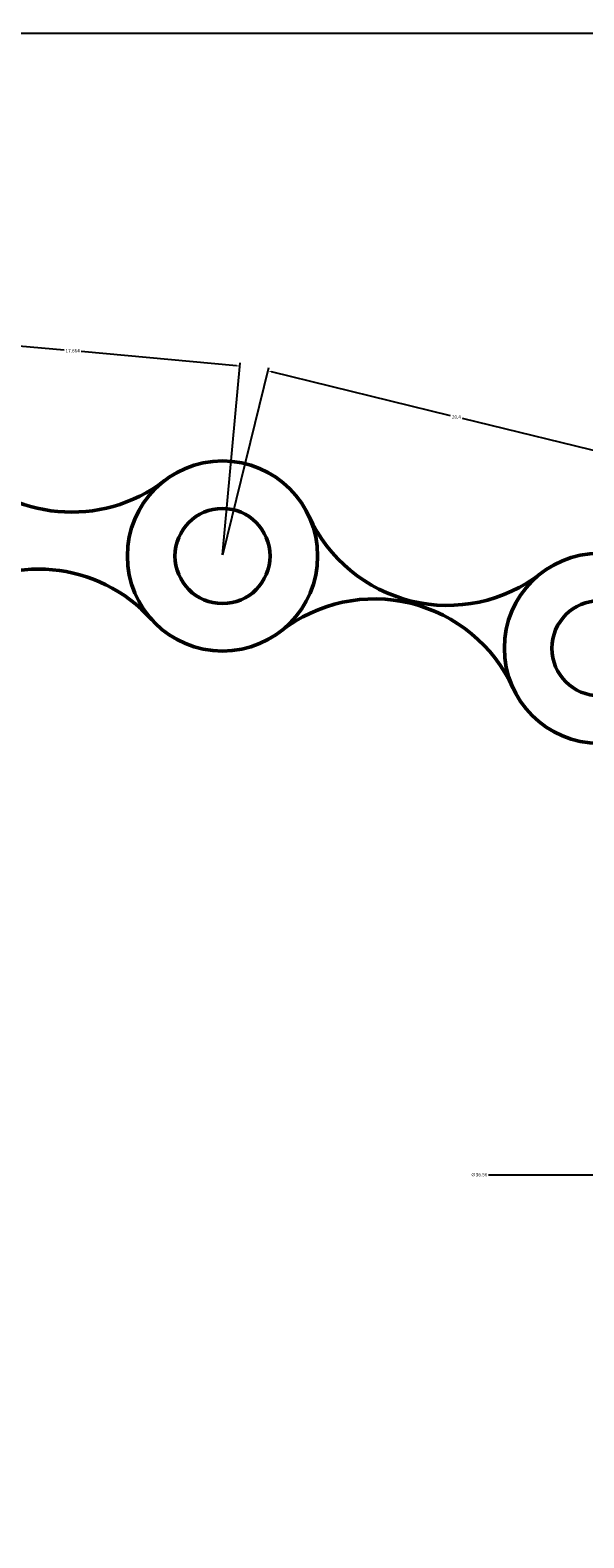
# Model space of a CAD drawing. Units: inches. Extents: x 413 to 622, y 326 to 447.
# Tile 11 of 15: x 539 to 568, y 367 to 447. Entities that reach past the tile are written whole.
import ezdxf

# ---------------------------------------------------------------- set-up
doc = ezdxf.new("R2010")
doc.units = ezdxf.units.IN
doc.header["$MEASUREMENT"] = 0
doc.layers.add('M-DIMS', color=2, linetype='Continuous', lineweight=18)
doc.layers.add('M-OUTL', color=7, linetype='Continuous', lineweight=50)
doc.styles.get("Standard").update_dxf_attribs({"font": 'arial.ttf'})
doc.dimstyles.get("Standard").update_dxf_attribs({"dimtxt": 0.18, "dimasz": 0.18, "dimexe": 0.18, "dimexo": 0.0625, "dimgap": 0.09, "dimtad": 0, "dimtih": 1, "dimtoh": 1, "dimdec": 4, "dimzin": 0, "dimdsep": 46, "dimtxsty": 'Standard', "dimcen": 0.09, "dimadec": 0, "dimazin": 0, "dimtfac": 1, "dimtdec": 4, "dimtofl": 0, "dimtmove": 0, "dimatfit": 3, "dimfxl": 1, "dimtolj": 1, "dimtzin": 0, "dimarcsym": 0})

# ---------------------------------------------------------------- blocks, each defined once
blk = doc.blocks.new('CHAIN-ROLLER-PIN')
for radius in [5, 2.5]:
    blk.add_circle((5, 5), radius)
blk = doc.blocks.new('CHAIN-LINK-WAIST-P17_664')
for centre, start, end in [((6.624, 13.651), 221.93853, 307.52912), ((4.873, -5.347), 41.93853, 127.52912)]:
    blk.add_arc(centre, 8, start, end)
blk = doc.blocks.new('CHAIN-LINK-WAIST-P20_400')
for centre, start, end in [((8.752, 12.333), 204.55472, 307.92191), ((4.917, -3.325), 24.55472, 127.92191)]:
    blk.add_arc(centre, 8, start, end)
blk = doc.blocks.new('*D11')
at = {"layer": 'Defpoints', "color": 0, "transparency": 16777216}
for p in [(621.66, 446.422), (621.66, 388.074), (423.314, 378.888)]:
    blk.add_point(p, dxfattribs=at)
at = {"layer": 'M-DIMS', "color": 0, "lineweight": -2, "transparency": 16777216}
for p, q in [((423.314, 378.95), (423.314, 446.602)), ((621.66, 388.137), (621.66, 446.602)), ((423.494, 446.422), (522.031, 446.422)), ((621.48, 446.422), (522.943, 446.422))]:
    blk.add_line(p, q, dxfattribs=at)
at = {"layer": 'M-DIMS', "color": 0, "transparency": 16777216}
for points in [[(423.494, 446.452), (423.494, 446.392), (423.314, 446.422)], [(621.48, 446.452), (621.48, 446.392), (621.66, 446.422)]]:
    blk.add_solid(points, dxfattribs=at)
at = {"layer": 'M-DIMS', "color": 0, "transparency": 16777216, "insert": (522.487, 446.422), "char_height": 0.18, "attachment_point": 5}
blk.add_mtext('\\A1;198.35', dxfattribs=at)
blk = doc.blocks.new('*D12')
at = {"layer": 'Defpoints', "color": 0, "transparency": 16777216}
for p in [(472.684, 386.392), (592.684, 386.392), (592.684, 326.361)]:
    blk.add_point(p, dxfattribs=at)
at = {"layer": 'M-DIMS', "color": 0, "lineweight": -2, "transparency": 16777216}
for p, q in [((472.684, 386.329), (472.684, 326.181)), ((592.684, 386.329), (592.684, 326.181)), ((472.864, 326.361), (532.404, 326.361)), ((592.504, 326.361), (532.964, 326.361))]:
    blk.add_line(p, q, dxfattribs=at)
at = {"layer": 'M-DIMS', "color": 0, "transparency": 16777216}
for points in [[(472.864, 326.391), (472.864, 326.331), (472.684, 326.361)], [(592.504, 326.391), (592.504, 326.331), (592.684, 326.361)]]:
    blk.add_solid(points, dxfattribs=at)
at = {"layer": 'M-DIMS', "color": 0, "transparency": 16777216, "insert": (532.684, 326.361), "char_height": 0.18, "attachment_point": 5}
blk.add_mtext('\\A1;120', dxfattribs=at)
blk = doc.blocks.new('*D20')
at = {"layer": 'Defpoints', "color": 0, "transparency": 16777216}
for p in [(550.373, 428.926), (531.863, 420.559), (549.452, 418.938)]:
    blk.add_point(p, dxfattribs=at)
at = {"layer": 'M-DIMS', "color": 0, "lineweight": -2, "transparency": 16777216}
for p, q in [((531.869, 420.621), (532.8, 430.726)), ((532.963, 430.53), (541.124, 429.778)), ((550.194, 428.942), (542.033, 429.694)), ((549.458, 419), (550.39, 429.105))]:
    blk.add_line(p, q, dxfattribs=at)
at = {"layer": 'M-DIMS', "color": 0, "transparency": 16777216}
for points in [[(532.966, 430.56), (532.96, 430.501), (532.784, 430.547)], [(550.197, 428.972), (550.191, 428.912), (550.373, 428.926)]]:
    blk.add_solid(points, dxfattribs=at)
at = {"layer": 'M-DIMS', "color": 0, "transparency": 16777216, "insert": (541.578, 429.736), "char_height": 0.18, "attachment_point": 5}
blk.add_mtext('\\A1;17.664', dxfattribs=at)
blk = doc.blocks.new('*D21')
at = {"layer": 'Defpoints', "color": 0, "transparency": 16777216}
for p in [(571.652, 423.827), (549.452, 418.938), (569.266, 414.085)]:
    blk.add_point(p, dxfattribs=at)
at = {"layer": 'M-DIMS', "color": 0, "lineweight": -2, "transparency": 16777216}
for p, q in [((549.467, 418.998), (551.881, 428.855)), ((552.013, 428.637), (561.421, 426.333)), ((571.478, 423.87), (562.07, 426.174)), ((569.281, 414.145), (571.695, 424.002))]:
    blk.add_line(p, q, dxfattribs=at)
at = {"layer": 'M-DIMS', "color": 0, "transparency": 16777216}
for points in [[(552.02, 428.666), (552.006, 428.608), (551.838, 428.68)], [(571.485, 423.899), (571.47, 423.841), (571.652, 423.827)]]:
    blk.add_solid(points, dxfattribs=at)
at = {"layer": 'M-DIMS', "color": 0, "transparency": 16777216, "insert": (561.745, 426.254), "char_height": 0.18, "attachment_point": 5}
blk.add_mtext('\\A1;20.4', dxfattribs=at)
blk = doc.blocks.new('*D25')
at = {"layer": 'Defpoints', "color": 0, "transparency": 16777216}
for p in [(574.404, 386.392), (610.964, 386.391)]:
    blk.add_point(p, dxfattribs=at)
at = {"layer": 'M-DIMS', "color": 0, "lineweight": -2, "transparency": 16777216}
for p, q in [((563.436, 386.392), (574.224, 386.392)), ((592.594, 386.392), (592.774, 386.392)), ((592.684, 386.302), (592.684, 386.482))]:
    blk.add_line(p, q, dxfattribs=at)
at = {"layer": 'M-DIMS', "color": 0, "transparency": 16777216}
blk.add_solid([(574.224, 386.422), (574.224, 386.362), (574.404, 386.392)], dxfattribs=at)
at = {"layer": 'M-DIMS', "color": 0, "transparency": 16777216, "insert": (562.944, 386.392), "char_height": 0.18, "attachment_point": 5}
blk.add_mtext('\\A1;∅36.56', dxfattribs=at)

msp = doc.modelspace()

# ---------------------------------------------------------------- block references
at = {"layer": 'M-OUTL'}
for name, p in [('CHAIN-LINK-WAIST-P17_664', (534.909, 415.596)), ('CHAIN-ROLLER-PIN', (544.4528, 413.938)), ('CHAIN-LINK-WAIST-P20_400', (552.525, 412.007)), ('CHAIN-ROLLER-PIN', (564.2668, 409.0853))]:
    msp.add_blockref(name, p, dxfattribs=at)

# ---------------------------------------------------------------- dimensions: what is measured, and where the dimension line sits
at = {"layer": 'M-DIMS'}
for base, p1, p2, override, picture, middle in [((621.66, 446.422), (423.3136, 378.8878), (621.66, 388.0741), {"dimdec": 2, "dimlfac": 1, "dimrnd": 0, "dimzin": 0, "dimdsep": 46, "dimlunit": 2}, '*D11', (522.4868, 446.422)), ((592.6836, 326.361), (472.6836, 386.3915), (592.6836, 386.3915), {"dimdec": 0, "dimlfac": 1, "dimrnd": 0, "dimzin": 0, "dimdsep": 46, "dimlunit": 2}, '*D12', (532.6836, 326.361))]:
    dim = msp.add_linear_dim(base=base, p1=p1, p2=p2, dimstyle='Standard', override=override, dxfattribs=at)
    dim.commit()
    dim.dimension.update_dxf_attribs({"geometry": picture, "text_midpoint": middle})
for base, p1, p2, angle, override, picture, middle in [((550.373, 428.9257), (531.863, 420.5588), (549.4524, 418.9375), 354.733826, {"dimdec": 3, "dimlfac": 1, "dimrnd": 0, "dimzin": 0, "dimdsep": 46, "dimlunit": 2}, '*D20', (541.5783, 429.7363)), ((571.6524, 423.8274), (549.4524, 418.9375), (569.2663, 414.0848), 346.238314, {"dimdec": 1, "dimlfac": 1, "dimrnd": 0, "dimzin": 0, "dimdsep": 46, "dimlunit": 2}, '*D21', (561.7455, 426.2537))]:
    dim = msp.add_linear_dim(base=base, p1=p1, p2=p2, angle=angle, dimstyle='Standard', override=override, dxfattribs=at)
    dim.commit()
    dim.dimension.update_dxf_attribs({"geometry": picture, "text_midpoint": middle})
dim = msp.add_diameter_dim_2p(p1=(610.9636, 386.391), p2=(574.4036, 386.392), dimstyle='Standard', override={"dimdec": 2, "dimlfac": 1, "dimrnd": 0, "dimzin": 0, "dimdsep": 46, "dimlunit": 2}, dxfattribs=at)
dim.commit()
dim.dimension.update_dxf_attribs({"geometry": '*D25', "text_midpoint": (563.4356, 386.3923), "dimtype": 163})

doc.saveas('drawing.dxf')
